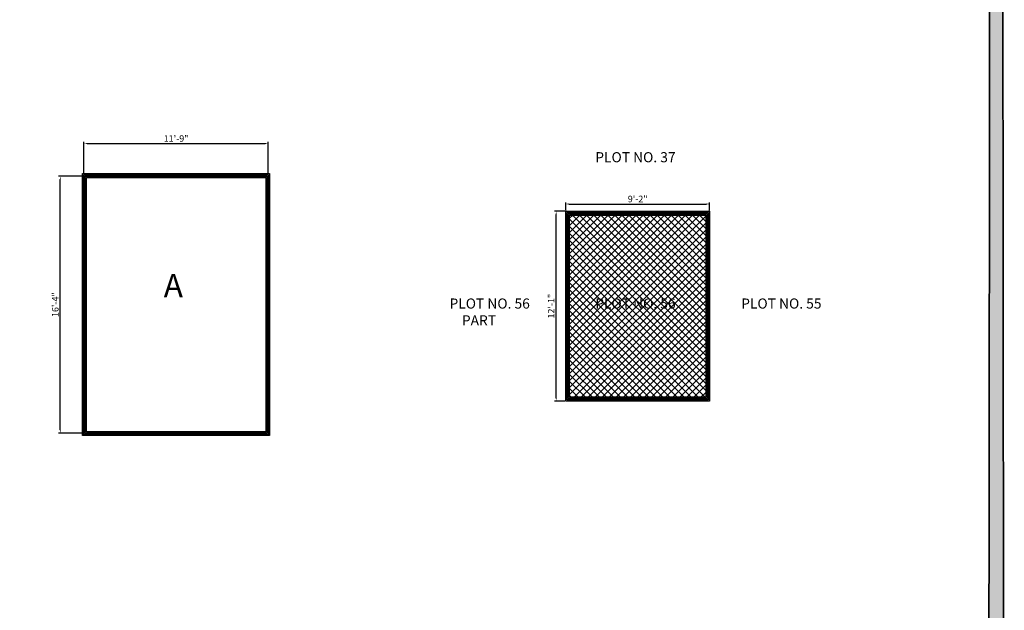
# Model space of a CAD drawing. Units: inches. Extents: x 1804 to 3296, y 909 to 2477.
# Tile 25 of 31: x 2543 to 3296, y 1449 to 1900. Entities that reach past the tile are written whole.
import ezdxf

# ---------------------------------------------------------------- set-up
doc = ezdxf.new("R2010")
doc.units = ezdxf.units.IN
for name, color, linetype, lineweight in [('A-ANNO-DIMS', 2, 'Continuous', 18), ('A-ANNO-TTLB', 156, 'Continuous', 35), ('A-WALL-PATT', 10, 'Continuous', 13), ('C-PROP', 7, 'Continuous', 25), ('C-PROP-PATT', 85, 'Continuous', 13), ('TEXT', 190, 'Continuous', 18)]:
    doc.layers.add(name, color=color, linetype=linetype, lineweight=lineweight)
doc.styles.get("Standard").update_dxf_attribs({"font": 'arial.ttf'})
doc.dimstyles.new('ISO-25', dxfattribs={"dimtxt": 5, "dimasz": 2.5, "dimexe": 1.25, "dimexo": 0.625, "dimtad": 1, "dimdec": 0, "dimlunit": 4, "dimtxsty": 'Standard', "dimcen": 2.5, "dimadec": 0, "dimazin": 0, "dimtfac": 1, "dimtdec": 0, "dimtmove": 0, "dimatfit": 3, "dimfxl": 1, "dimarcsym": 0})

# ---------------------------------------------------------------- blocks, each defined once
blk = doc.blocks.new('*D36')
at = {"layer": 'A-ANNO-DIMS', "color": 0, "lineweight": -2, "transparency": 16777216}
for p, q in [((2592.54, 1782.01), (2592.54, 1806.64)), ((2733.5, 1782.01), (2733.5, 1806.64)), ((2595.04, 1805.39), (2731, 1805.39))]:
    blk.add_line(p, q, dxfattribs=at)
at = {"layer": 'A-ANNO-DIMS', "color": 0, "lineweight": 100, "transparency": 16777216}
for points in [[(2595.04, 1805.81), (2595.04, 1804.97), (2592.54, 1805.39)], [(2731, 1805.81), (2731, 1804.97), (2733.5, 1805.39)]]:
    blk.add_solid(points, dxfattribs=at)
at = {"layer": 'Defpoints', "color": 0, "lineweight": 100, "transparency": 16777216}
for p in [(2733.5, 1805.39), (2592.54, 1781.39), (2733.5, 1781.39)]:
    blk.add_point(p, dxfattribs=at)
at = {"layer": 'A-ANNO-DIMS', "color": 0, "transparency": 16777216, "insert": (2663.02, 1808.57), "char_height": 5, "attachment_point": 5}
blk.add_mtext('11\'-9"', dxfattribs=at)
blk = doc.blocks.new('*D37')
at = {"layer": 'A-ANNO-DIMS', "color": 0, "lineweight": -2, "transparency": 16777216}
for p, q in [((2592.91, 1780.39), (2573.24, 1780.39)), ((2574.49, 1586.59), (2574.49, 1777.89)), ((2592.91, 1584.09), (2573.24, 1584.09))]:
    blk.add_line(p, q, dxfattribs=at)
at = {"layer": 'A-ANNO-DIMS', "color": 0, "lineweight": 100, "transparency": 16777216}
for points in [[(2574.08, 1777.89), (2574.91, 1777.89), (2574.49, 1780.39)], [(2574.08, 1586.59), (2574.91, 1586.59), (2574.49, 1584.09)]]:
    blk.add_solid(points, dxfattribs=at)
at = {"layer": 'Defpoints', "color": 0, "lineweight": 100, "transparency": 16777216}
for p in [(2574.49, 1780.39), (2593.54, 1780.39), (2593.54, 1584.09)]:
    blk.add_point(p, dxfattribs=at)
at = {"layer": 'A-ANNO-DIMS', "color": 0, "transparency": 16777216, "insert": (2571.31, 1682.24), "char_height": 5, "attachment_point": 5, "rotation": 90}
blk.add_mtext('16\'-4"', dxfattribs=at)
blk = doc.blocks.new('*D38')
at = {"layer": 'A-ANNO-DIMS', "color": 0, "lineweight": -2, "transparency": 16777216}
for p, q in [((2960.24, 1753.62), (2952.33, 1753.62)), ((2953.58, 1610.99), (2953.58, 1751.12)), ((2960.24, 1608.49), (2952.33, 1608.49))]:
    blk.add_line(p, q, dxfattribs=at)
at = {"layer": 'A-ANNO-DIMS', "color": 0, "lineweight": 100, "transparency": 16777216}
for points in [[(2953.16, 1751.12), (2954, 1751.12), (2953.58, 1753.62)], [(2953.16, 1610.99), (2954, 1610.99), (2953.58, 1608.49)]]:
    blk.add_solid(points, dxfattribs=at)
at = {"layer": 'Defpoints', "color": 0, "lineweight": 100, "transparency": 16777216}
for p in [(2953.58, 1753.62), (2960.87, 1753.62), (2960.87, 1608.49)]:
    blk.add_point(p, dxfattribs=at)
at = {"layer": 'A-ANNO-DIMS', "color": 0, "transparency": 16777216, "insert": (2950.44, 1681.06), "char_height": 5, "attachment_point": 5, "rotation": 90}
blk.add_mtext('12\'-1"', dxfattribs=at)
blk = doc.blocks.new('*D39')
at = {"layer": 'A-ANNO-DIMS', "color": 0, "lineweight": -2, "transparency": 16777216}
for p, q in [((2960.87, 1754.25), (2960.87, 1760.42)), ((2963.37, 1759.17), (3068.4, 1759.17)), ((3070.9, 1754.25), (3070.9, 1760.42))]:
    blk.add_line(p, q, dxfattribs=at)
at = {"layer": 'A-ANNO-DIMS', "color": 0, "lineweight": 100, "transparency": 16777216}
for points in [[(2963.37, 1759.59), (2963.37, 1758.76), (2960.87, 1759.17)], [(3068.4, 1759.59), (3068.4, 1758.76), (3070.9, 1759.17)]]:
    blk.add_solid(points, dxfattribs=at)
at = {"layer": 'Defpoints', "color": 0, "lineweight": 100, "transparency": 16777216}
for p in [(3070.9, 1759.17), (2960.87, 1753.62), (3070.9, 1753.62)]:
    blk.add_point(p, dxfattribs=at)
at = {"layer": 'A-ANNO-DIMS', "color": 0, "transparency": 16777216, "insert": (3015.89, 1762.35), "char_height": 5, "attachment_point": 5}
blk.add_mtext('9\'-2"', dxfattribs=at)

msp = doc.modelspace()

# ---------------------------------------------------------------- hatches: boundary and pattern name
at = {"layer": 'A-ANNO-TTLB'}
h = msp.add_hatch(color=256, dxfattribs=at)
h.dxf.hatch_style = 1
h.paths.add_polyline_path([(3294.53, 2476.54), (1803.79, 2476.54), (1805.43, 909.47), (3296.17, 909.47)])
h.paths.add_polyline_path([(1811, 914.33), (1812.79, 2467.54), (3285.53, 2467.54), (3283.74, 914.33)], flags=16)
h.paths.add_polyline_path([(1925.58, 1062.77), (1925.58, 1138.07), (1925.58, 1539.88), (1925.58, 1793.38), (1925.58, 1830.04), (2325.54, 1830.04), (2325.54, 1793.38), (2325.54, 1586.42), (2325.54, 1138.07), (2325.54, 1062.77)], flags=0)
h.paths.add_polyline_path([(1997.22, 1029.4), (2008.85, 1037.96), (2008.85, 1020.84)], flags=0)
h.paths.add_polyline_path([(1934.58, 1138.07), (1934.58, 1147.07), (2078.77, 1147.07), (2078.77, 1138.07), (2060.94, 1138.07)], flags=0)
h.paths.add_polyline_path([(1944.35, 1138.07), (1944.35, 1147.07), (2056.05, 1147.07), (2056.05, 1138.07)], flags=0)
h.paths.add_polyline_path([(2222.24, 1037.96), (2233.87, 1029.4), (2222.24, 1020.84)], flags=0)
h.paths.add_polyline_path([(2061.94, 1139.07), (2061.94, 1146.07), (2077.77, 1146.07), (2077.77, 1139.07)], flags=0)
h.paths.add_polyline_path([(2149.58, 1138.07), (2149.58, 1269.44), (2158.58, 1269.44), (2158.58, 1326.69), (2149.58, 1326.69), (2149.58, 1340.94), (2139.6, 1340.94), (2139.6, 1434.25), (2149.58, 1434.25), (2149.58, 1447.36), (2158.58, 1447.36), (2158.58, 1423.87), (2158.58, 1408.06), (2198.46, 1408.06), (2198.46, 1412.56), (2282.65, 1412.56), (2282.65, 1465.94), (2316.54, 1465.94), (2316.54, 1590.92), (2192.86, 1590.92), (2192.86, 1595.3), (2291.17, 1595.3), (2291.17, 1590.92), (2316.54, 1590.92), (2316.54, 1784.38), (2300.24, 1784.38), (2300.24, 1757.47), (2268, 1757.47), (2268, 1681.04), (2180.87, 1681.04), (2180.87, 1757.47), (2148.63, 1757.47), (2148.63, 1784.38), (2119.08, 1784.38), (2119.08, 1585.58), (2114.58, 1585.58), (2114.58, 1784.38), (2064.11, 1784.38), (2046.28, 1784.38), (2046.28, 1760.38), (1958.58, 1760.38), (1958.58, 1664.38), (1934.58, 1664.38), (1934.58, 1784.38), (1934.58, 1793.38), (2046.28, 1793.38), (2064.11, 1793.38), (2119.08, 1793.38), (2230.78, 1793.38), (2230.78, 1784.38), (2268, 1784.38), (2300.24, 1784.38), (2316.54, 1784.38), (2316.54, 1590.92), (2316.54, 1373.73), (2316.54, 1138.07)], flags=0)
h.paths.add_polyline_path([(2209.19, 1166.63), (2209.19, 1175.63), (2158.58, 1175.63), (2209.19, 1223.63), (2209.19, 1231.63), (2183.88, 1231.63), (2183.88, 1301.66), (2242.59, 1301.66), (2242.59, 1326.69), (2316.54, 1326.69), (2272.59, 1271.63), (2272.59, 1223.63), (2316.54, 1175.63), (2272.59, 1175.63), (2272.59, 1166.63)], flags=0)
h.paths.add_polyline_path([(1947.77, 1345.22), (1947.77, 1457.48), (1991.2, 1457.48), (1991.2, 1451.7), (1991.2, 1352.18), (1991.2, 1345.22)], flags=0)
h.paths.add_polyline_path([(2209.19, 1271.63), (2262.59, 1271.63), (2262.59, 1311.85), (2272.59, 1301.66), (2272.59, 1271.63), (2269.92, 1269.63), (2270.59, 1269.63), (2270.59, 1225.63), (2211.19, 1225.63), (2211.19, 1269.63), (2211.86, 1269.63)], flags=0)
h.paths.add_polyline_path([(2000.34, 1378.21), (2000.34, 1429.71), (2025.22, 1429.71), (2025.22, 1378.21)], flags=0)
h.paths.add_polyline_path([(2001.34, 1379.21), (2001.34, 1428.71), (2024.22, 1428.71), (2024.22, 1379.21)], flags=0)
h.paths.add_polyline_path([(2012.34, 1390.21), (2012.34, 1417.71), (2013.22, 1417.71), (2013.22, 1390.21)], flags=0)
h.paths.add_polyline_path([(2237.56, 1331.19), (2237.56, 1340.18), (2238.62, 1340.18), (2238.62, 1386.84), (2241.04, 1386.84), (2242.06, 1386.84), (2242.06, 1408.06), (2316.54, 1331.19)], flags=0)
h.paths.add_polyline_path([(1953.73, 1464.35), (1953.73, 1498.59), (1981.74, 1498.59), (1981.74, 1464.35)], flags=0)
h.paths.add_polyline_path([(1987.63, 1462.08), (1987.63, 1500.95), (2104.07, 1500.95), (2104.07, 1462.08), (2099.27, 1462.08), (1993.6, 1462.08)], flags=0)
h.paths.add_polyline_path([(1956.06, 1481.47, -1), (1979.41, 1481.47, -1)], flags=0)
edge = h.paths.add_edge_path(flags=0)
edge.add_ellipse((2299.53, 1438.37), major_axis=(0.31, 21.36), ratio=0.670333, start_angle=0, end_angle=360)
h.paths.add_polyline_path([(2297.39, 1438.37, -1), (2301.67, 1438.37, -1)], flags=0)
h.paths.add_polyline_path([(2591.54, 1163.23), (2591.54, 1179.38), (2591.54, 1379.68), (2591.54, 1395.84), (2734.5, 1395.84), (2734.5, 1379.68), (2734.5, 1179.38), (2734.5, 1163.23)], flags=0)
h.paths.add_polyline_path([(2592.54, 1164.23), (2592.54, 1166.23), (2733.5, 1166.23), (2733.5, 1164.23)], flags=0)
h.paths.add_polyline_path([(2592.54, 1180.38), (2592.54, 1378.68), (2733.5, 1378.68), (2733.5, 1180.38)], flags=0)
h.paths.add_polyline_path([(2593.54, 1181.38), (2593.54, 1377.68), (2732.5, 1377.68), (2732.5, 1181.38)], flags=0)
h.paths.add_polyline_path([(2594.54, 1182.38), (2594.54, 1376.68), (2731.5, 1376.68), (2731.5, 1182.38)], flags=0)
h.paths.add_polyline_path([(1936.95, 1697.46), (1936.95, 1736.46), (1955.41, 1736.46), (1955.41, 1697.46)], flags=0)
h.paths.add_polyline_path([(1938.48, 1718.36), (1938.48, 1734.92), (1953.65, 1734.92), (1953.65, 1718.36)], flags=0)
h.paths.add_polyline_path([(1944.75, 1726.64, -1), (1947.37, 1726.64, -1)], flags=0)
h.paths.add_polyline_path([(2592.54, 1394.84), (2733.5, 1394.84), (2733.5, 1392.84), (2592.54, 1392.84)], flags=0)
h.paths.add_polyline_path([(1976.61, 1762.5), (1976.61, 1781.44), (2012.79, 1781.44), (2012.79, 1762.5)], flags=0)
h.paths.add_polyline_path([(1979.57, 1771.97, -1), (1991.39, 1771.97, -1)], flags=0)
h.paths.add_polyline_path([(1995.36, 1771.97, -1), (2007.18, 1771.97, -1)], flags=0)
h.paths.add_polyline_path([(2251.51, 1744.53), (2268, 1730.05), (2251.51, 1730.05)], flags=0)
h.paths.add_polyline_path([(2047.28, 1785.38), (2047.28, 1792.38), (2063.11, 1792.38), (2063.11, 1785.38)], flags=0)
h.paths.add_polyline_path([(2155.08, 1770.92, -1), (2174.42, 1770.92, -1)], flags=0)
h.paths.add_polyline_path([(2188.59, 1758.27), (2188.59, 1772.81), (2222.3, 1772.81), (2222.3, 1758.27)], flags=0)
h.paths.add_polyline_path([(2223.97, 1758.27), (2223.97, 1772.81), (2257.68, 1772.81), (2257.68, 1758.27)], flags=0)
h.paths.add_polyline_path([(2274.45, 1770.92, -1), (2293.8, 1770.92, -1)], flags=0)
h.paths.add_polyline_path([(2591.54, 1582.09), (2591.54, 1782.39), (2734.5, 1782.39), (2734.5, 1582.09)], flags=0)
h.paths.add_polyline_path([(2592.54, 1583.09), (2592.54, 1781.39), (2733.5, 1781.39), (2733.5, 1583.09)], flags=0)
h.paths.add_polyline_path([(2593.54, 1584.09), (2593.54, 1780.39), (2732.5, 1780.39), (2732.5, 1584.09)], flags=0)
h.paths.add_polyline_path([(2594.54, 1585.09), (2594.54, 1779.39), (2731.5, 1779.39), (2731.5, 1585.09)], flags=0)
h.paths.add_polyline_path([(1922.17, 1978.79), (1922.17, 2295.08), (1922.17, 2296.08), (2115.67, 2296.08), (2115.67, 2384.31), (2115.67, 2385.31), (2322.12, 2385.31), (2323.12, 2385.31), (2323.12, 1979.79), (2323.12, 1978.79), (1923.17, 1978.79)], flags=0)
h.paths.add_polyline_path([(1922.17, 1978.79), (1922.17, 2051.31), (1922.17, 2214.86), (1922.17, 2296.08), (2115.67, 2296.08), (2115.67, 2385.31), (2323.12, 2385.31), (2323.12, 2280.42), (2323.12, 1978.79), (2115.67, 1978.79)], flags=0)
h.paths.add_polyline_path([(1923.17, 1979.79), (1923.17, 2050.31), (2115.67, 2050.31), (2115.67, 2051.31), (1923.17, 2051.31), (1923.17, 2213.86), (1923.17, 2214.86), (1923.17, 2295.08), (1990.02, 2295.08), (1990.02, 2214.86), (1991.02, 2214.86), (1991.02, 2295.08), (2115.67, 2295.08), (2115.67, 1979.79), (2116.67, 1979.79), (2116.67, 2304.18), (2116.67, 2384.31), (2322.12, 2384.31), (2322.12, 2280.42), (2322.12, 1979.79), (2115.67, 1979.79)], flags=0)
h.paths.add_polyline_path([(2972.46, 1192.5), (2972.46, 1196.92), (2995.47, 1196.92), (2995.47, 1255.47), (2995.09, 1255.47), (2987.42, 1249.39), (2980.08, 1255.47), (2978.05, 1255.47), (2978.05, 1257.24), (2995.47, 1257.24), (2995.47, 1261.58), (3015.37, 1261.58), (3015.37, 1333.28), (3015.37, 1414.4), (3032.82, 1414.4), (3032.82, 1333.28), (3032.82, 1261.58), (3052.66, 1261.58), (3052.66, 1255.47), (3079.86, 1255.47), (3078.72, 1254.57), (3081.47, 1252.29), (3078.56, 1249.99), (3075.81, 1252.26), (3072.57, 1249.69), (3070.36, 1251.52), (3067.67, 1249.39), (3060.34, 1255.47), (3052.66, 1255.47), (3052.66, 1196.92), (3054.58, 1196.92), (3074, 1196.92), (3074, 1192.5), (3052.66, 1192.5), (2995.47, 1192.5)], flags=0)
h.paths.add_polyline_path([(2490.75, 1979.27), (2490.75, 1980.27), (2596.87, 1980.27), (2596.87, 2051.8), (2596.87, 2052.8), (2596.87, 2216.35), (2596.87, 2297.57), (2717.32, 2297.57), (2710.57, 2305.62), (2724.07, 2305.62), (2717.32, 2297.57), (2782.37, 2297.57), (2782.37, 2395.8), (3006.82, 2395.8), (3006.82, 1981.27), (3093.73, 1981.27), (3093.73, 1980.27), (3047.51, 1980.27), (3046.37, 1979.37), (3049.11, 1977.1), (3046.2, 1974.79), (3043.46, 1977.07), (3040.21, 1974.49), (3038, 1976.32), (3035.32, 1974.2), (3027.98, 1980.27), (2871.83, 1980.27), (2871.83, 1981.27), (2791.37, 1981.27), (2791.37, 2050.8), (2597.87, 2050.8), (2597.87, 1980.27), (2597.87, 1979.27), (2546.27, 1979.27), (2545.12, 1978.37), (2547.87, 1976.1), (2544.96, 1973.79), (2542.22, 1976.07), (2538.97, 1973.49), (2536.76, 1975.32), (2534.07, 1973.2), (2526.74, 1979.27)], flags=0)
h.paths.add_polyline_path([(2597.87, 2051.8), (2606.87, 2051.8), (2606.87, 2258.39), (2597.87, 2258.39), (2597.87, 2296.57), (2606.87, 2296.57), (2606.87, 2262.39), (2782.37, 2262.39), (2782.37, 2296.57), (2790.37, 2296.57), (2790.37, 2262.39), (2791.37, 2262.39), (2791.37, 2305.67), (2791.37, 2385.8), (2996.82, 2385.8), (2996.82, 2339.85), (3006.82, 2339.85), (3006.82, 2250.12), (2997.82, 2250.12), (2997.82, 1981.27), (2996.82, 1981.27), (2872.83, 1981.27), (2872.83, 1991.8), (2871.83, 1991.8), (2871.83, 2050.8), (2790.37, 2050.8), (2597.87, 2050.8)], flags=0)
h.paths.add_polyline_path([(2179.93, 2153.92), (2179.93, 2353.97), (2259.98, 2353.97), (2259.98, 2153.92)], flags=0)
h.paths.add_polyline_path([(2180.93, 2154.92), (2180.93, 2352.97), (2258.98, 2352.97), (2258.98, 2154.92)], flags=0)
h.paths.add_polyline_path([(2960.87, 1608.49), (2960.87, 1753.62), (3070.9, 1753.62), (3070.9, 1608.49)], flags=0)
h.paths.add_polyline_path([(2961.87, 1609.49), (2961.87, 1752.62), (3069.9, 1752.62), (3069.9, 1609.49)], flags=0)
h.paths.add_polyline_path([(2962.87, 1610.49), (2962.87, 1751.62), (3068.9, 1751.62), (3068.9, 1610.49)], flags=0)
h.paths.add_polyline_path([(2963.87, 1611.49), (2963.87, 1750.62), (3067.9, 1750.62), (3067.9, 1611.49)], flags=0)
h.paths.add_polyline_path([(2782.37, 2051.8), (2782.37, 2216.32), (2791.37, 2216.32), (2791.37, 2051.8), (2872.83, 2051.8), (2872.83, 2068.56), (2884.67, 2068.56), (2884.67, 2085.33), (2896.51, 2085.33), (2896.51, 2102.09), (2908.36, 2102.09), (2908.36, 2118.85), (2920.2, 2118.85), (2920.2, 2135.62), (2932.05, 2135.62), (2932.05, 2145.3), (2925.08, 2145.3), (2925.08, 2203.2), (2996.82, 2203.2), (2996.82, 2145.3), (2953.82, 2145.3), (2872.83, 2051.8), (2790.37, 2051.8)], flags=0)
h.paths.add_polyline_path([(2717.32, 2238.65), (2710.57, 2246.7), (2724.07, 2246.7)], flags=0)
h.paths.add_polyline_path([(2003.09, 1122.79), (2017.16, 1122.79), (2017.16, 1138.74), (2003.09, 1138.74)], flags=8)
h.paths.add_polyline_path([(2174.76, 1792.72), (2188.83, 1792.72), (2188.83, 1808.66), (2174.76, 1808.66)], flags=8)
h.paths.add_polyline_path([(1987.95, 1792.51), (2002.02, 1792.51), (2002.02, 1808.45), (1987.95, 1808.45)], flags=8)
h.paths.add_polyline_path([(2148.79, 1289.26), (2160.46, 1289.26), (2160.46, 1305.2), (2148.79, 1305.2)], flags=8)
h.paths.add_polyline_path([(2115.36, 1133.57), (2127.04, 1133.57), (2127.04, 1149.51), (2115.36, 1149.51)], flags=8)
h.paths.add_polyline_path([(2237.58, 1421.48), (2249.25, 1421.48), (2249.25, 1437.43), (2237.58, 1437.43)], flags=8)
h.paths.add_polyline_path([(2134.99, 1584.32), (2146.66, 1584.32), (2146.66, 1600.26), (2134.99, 1600.26)], flags=8)
h.paths.add_polyline_path([(2101.95, 1557.31), (2113.62, 1557.31), (2113.62, 1573.25), (2101.95, 1573.25)], flags=8)
h.paths.add_polyline_path([(2937.85, 1156.77), (3120.41, 1156.77), (3120.41, 1185.72), (2937.85, 1185.72)], flags=8)
h.paths.add_polyline_path([(2980.71, 1786.71), (3050.06, 1786.71), (3050.06, 1802.66), (2980.71, 1802.66)], flags=8)
h.paths.add_polyline_path([(2869.28, 1661.96), (2938.62, 1661.96), (2938.62, 1690.8), (2869.28, 1690.8)], flags=8)
h.paths.add_polyline_path([(3092.27, 1674.86), (3161.62, 1674.86), (3161.62, 1690.8), (3092.27, 1690.8)], flags=8)
h.paths.add_polyline_path([(2980.71, 1674.86), (3050.06, 1674.86), (3050.06, 1690.8), (2980.71, 1690.8)], flags=8)
h.paths.add_polyline_path([(2649.07, 1678.23), (2674.53, 1678.23), (2674.53, 1714.76), (2649.07, 1714.76)], flags=8)
h.paths.add_polyline_path([(2530.84, 1981.63), (2549.13, 1981.63), (2549.13, 1997.57), (2530.84, 1997.57)], flags=8)
h.paths.add_polyline_path([(3031.29, 1981.77), (3049.58, 1981.77), (3049.58, 1997.71), (3031.29, 1997.71)], flags=8)
h.paths.add_polyline_path([(2715.38, 1911.9), (2851.54, 1911.9), (2851.54, 1940.85), (2715.38, 1940.85)], flags=8)
h.paths.add_polyline_path([(2015.23, 1927.36), (2205.42, 1927.36), (2205.42, 1956.3), (2015.23, 1956.3)], flags=8)
h.paths.add_polyline_path([(2671.84, 2057.84), (2702.75, 2057.84), (2702.75, 2073.79), (2671.84, 2073.79)], flags=8)
h.paths.add_polyline_path([(2678.5, 2316.52), (2765.26, 2316.52), (2765.26, 2332.46), (2678.5, 2332.46)], flags=8)
h.paths.add_polyline_path([(2678.48, 2271.96), (2736.41, 2271.96), (2736.41, 2287.9), (2678.48, 2287.9)], flags=8)
h.paths.add_polyline_path([(2019.2, 972.79), (2243.21, 972.79), (2243.21, 1001.74), (2019.2, 1001.74)], flags=8)
h.paths.add_polyline_path([(2097.06, 1021.56), (2132.16, 1021.56), (2132.16, 1037.51), (2097.06, 1037.51)], flags=8)
h.paths.add_polyline_path([(2182.47, 1360.48), (2207.35, 1360.48), (2207.35, 1376.42), (2182.47, 1376.42)], flags=8)
h.paths.add_polyline_path([(2261.12, 1361.77), (2295.01, 1361.77), (2295.01, 1377.71), (2261.12, 1377.71)], flags=8)
h.paths.add_polyline_path([(2245.75, 1511.51), (2278.44, 1511.51), (2278.44, 1527.46), (2245.75, 1527.46)], flags=8)
h.paths.add_polyline_path([(1991.16, 1296.29), (2060.51, 1296.29), (2060.51, 1312.23), (1991.16, 1312.23)], flags=8)
h.paths.add_polyline_path([(2187, 1651.35), (2246.71, 1651.35), (2246.71, 1667.29), (2187, 1667.29)], flags=8)
h.paths.add_polyline_path([(1976.49, 1684.81), (2068.63, 1684.81), (2068.63, 1700.76), (1976.49, 1700.76)], flags=8)
at = {"layer": 'A-WALL-PATT'}
h = msp.add_hatch(color=256, dxfattribs=at)
h.dxf.hatch_style = 1
h.paths.add_polyline_path([(2119.08, 1544.38), (1925.58, 1544.38), (1925.58, 1539.88), (2119.08, 1539.88)])
h.paths.add_polyline_path([(2119.08, 1545.58), (2114.58, 1545.58), (2114.58, 1544.38), (2119.08, 1544.38)])
h.paths.add_polyline_path([(1965.87, 1658.79), (1965.87, 1679.09), (1955.57, 1679.09), (1955.57, 1658.79)], flags=9)
h.paths.add_polyline_path([(2293.18, 1677.29), (2293.18, 1697.58), (2282.88, 1697.58), (2282.88, 1677.29)], flags=9)
h.paths.add_polyline_path([(2271.13, 1545.23), (2287.53, 1545.23), (2287.53, 1555.53), (2271.13, 1555.53)], flags=9)
h.paths.add_polyline_path([(2303.26, 1488.52), (2303.26, 1508.82), (2292.95, 1508.82), (2292.95, 1488.52)], flags=9)
h.paths.add_polyline_path([(2271.13, 1393.15), (2287.53, 1393.15), (2287.53, 1403.45), (2271.13, 1403.45)], flags=9)
h.paths.add_polyline_path([(2306.48, 1361.45), (2306.48, 1377.86), (2296.18, 1377.86), (2296.18, 1361.45)], flags=9)
h.paths.add_polyline_path([(2174.54, 1361.45), (2174.54, 1377.86), (2164.23, 1377.86), (2164.23, 1361.45)], flags=9)
h.paths.add_polyline_path([(1968.21, 1333.34), (1968.21, 1353.64), (1957.91, 1353.64), (1957.91, 1333.34)], flags=9)
h.paths.add_polyline_path([(2003.09, 1122.79), (2017.16, 1122.79), (2017.16, 1138.74), (2003.09, 1138.74)], flags=9)
h.paths.add_polyline_path([(2174.76, 1792.72), (2188.83, 1792.72), (2188.83, 1808.66), (2174.76, 1808.66)], flags=9)
h.paths.add_polyline_path([(1987.95, 1792.51), (2002.02, 1792.51), (2002.02, 1808.45), (1987.95, 1808.45)], flags=9)
h.paths.add_polyline_path([(2148.79, 1289.26), (2160.46, 1289.26), (2160.46, 1305.2), (2148.79, 1305.2)], flags=9)
h.paths.add_polyline_path([(2115.36, 1133.57), (2127.04, 1133.57), (2127.04, 1149.51), (2115.36, 1149.51)], flags=9)
h.paths.add_polyline_path([(2237.58, 1421.48), (2249.25, 1421.48), (2249.25, 1437.43), (2237.58, 1437.43)], flags=9)
h.paths.add_polyline_path([(2134.99, 1584.32), (2146.66, 1584.32), (2146.66, 1600.26), (2134.99, 1600.26)], flags=9)
h.paths.add_polyline_path([(2101.95, 1557.31), (2113.62, 1557.31), (2113.62, 1573.25), (2101.95, 1573.25)], flags=9)
h.paths.add_polyline_path([(2937.85, 1156.77), (3120.41, 1156.77), (3120.41, 1185.72), (2937.85, 1185.72)], flags=9)
h.paths.add_polyline_path([(2980.71, 1786.71), (3050.06, 1786.71), (3050.06, 1802.66), (2980.71, 1802.66)], flags=9)
h.paths.add_polyline_path([(2869.28, 1661.96), (2938.62, 1661.96), (2938.62, 1690.8), (2869.28, 1690.8)], flags=9)
h.paths.add_polyline_path([(3092.27, 1674.86), (3161.62, 1674.86), (3161.62, 1690.8), (3092.27, 1690.8)], flags=9)
h.paths.add_polyline_path([(2980.71, 1674.86), (3050.06, 1674.86), (3050.06, 1690.8), (2980.71, 1690.8)], flags=9)
h.paths.add_polyline_path([(2649.07, 1678.23), (2674.53, 1678.23), (2674.53, 1714.76), (2649.07, 1714.76)], flags=9)
h.paths.add_polyline_path([(2530.84, 1981.63), (2549.13, 1981.63), (2549.13, 1997.57), (2530.84, 1997.57)], flags=9)
h.paths.add_polyline_path([(3031.29, 1981.77), (3049.58, 1981.77), (3049.58, 1997.71), (3031.29, 1997.71)], flags=9)
h.paths.add_polyline_path([(2715.38, 1911.9), (2851.54, 1911.9), (2851.54, 1940.85), (2715.38, 1940.85)], flags=9)
h.paths.add_polyline_path([(2015.23, 1927.36), (2205.42, 1927.36), (2205.42, 1956.3), (2015.23, 1956.3)], flags=9)
h.paths.add_polyline_path([(2671.84, 2057.84), (2702.75, 2057.84), (2702.75, 2073.79), (2671.84, 2073.79)], flags=9)
h.paths.add_polyline_path([(2678.5, 2316.52), (2765.26, 2316.52), (2765.26, 2332.46), (2678.5, 2332.46)], flags=9)
h.paths.add_polyline_path([(2678.48, 2271.96), (2736.41, 2271.96), (2736.41, 2287.9), (2678.48, 2287.9)], flags=9)
h.paths.add_polyline_path([(2019.2, 972.79), (2243.21, 972.79), (2243.21, 1001.74), (2019.2, 1001.74)], flags=9)
h.paths.add_polyline_path([(2097.06, 1021.56), (2132.16, 1021.56), (2132.16, 1037.51), (2097.06, 1037.51)], flags=9)
h.paths.add_polyline_path([(2182.47, 1360.48), (2207.35, 1360.48), (2207.35, 1376.42), (2182.47, 1376.42)], flags=9)
h.paths.add_polyline_path([(2261.12, 1361.77), (2295.01, 1361.77), (2295.01, 1377.71), (2261.12, 1377.71)], flags=9)
h.paths.add_polyline_path([(2245.75, 1511.51), (2278.44, 1511.51), (2278.44, 1527.46), (2245.75, 1527.46)], flags=9)
h.paths.add_polyline_path([(1991.16, 1296.29), (2060.51, 1296.29), (2060.51, 1312.23), (1991.16, 1312.23)], flags=9)
h.paths.add_polyline_path([(2187, 1651.35), (2246.71, 1651.35), (2246.71, 1667.29), (2187, 1667.29)], flags=9)
h.paths.add_polyline_path([(1976.49, 1684.81), (2068.63, 1684.81), (2068.63, 1700.76), (1976.49, 1700.76)], flags=9)
h = msp.add_hatch(color=256, dxfattribs=at)
h.dxf.hatch_style = 1
h.paths.add_polyline_path([(2149.58, 1147.07), (2141.21, 1147.07), (2141.21, 1144.07), (2141.21, 1138.07), (2149.58, 1138.07)])
h.paths.add_polyline_path([(2101.21, 1144.07, -0.01877), (2101.32, 1147.07), (2078.77, 1147.07), (2078.77, 1138.07), (2101.21, 1138.07)])
h.paths.add_polyline_path([(2060.94, 1147.07), (2056.05, 1147.07), (2056.05, 1138.07), (2060.94, 1138.07)])
h.paths.add_polyline_path([(1944.35, 1147.07), (1934.58, 1147.07), (1934.58, 1138.07), (1944.35, 1138.07)])
h.paths.add_polyline_path([(2158.58, 1269.44), (2149.58, 1269.44), (2149.58, 1138.07), (2158.58, 1138.07)])
h.paths.add_polyline_path([(2003.09, 1122.79), (2017.16, 1122.79), (2017.16, 1138.74), (2003.09, 1138.74)], flags=9)
h.paths.add_polyline_path([(2174.76, 1792.72), (2188.83, 1792.72), (2188.83, 1808.66), (2174.76, 1808.66)], flags=9)
h.paths.add_polyline_path([(1987.95, 1792.51), (2002.02, 1792.51), (2002.02, 1808.45), (1987.95, 1808.45)], flags=9)
h.paths.add_polyline_path([(2148.79, 1289.26), (2160.46, 1289.26), (2160.46, 1305.2), (2148.79, 1305.2)], flags=9)
h.paths.add_polyline_path([(2115.36, 1133.57), (2127.04, 1133.57), (2127.04, 1149.51), (2115.36, 1149.51)], flags=9)
h.paths.add_polyline_path([(2237.58, 1421.48), (2249.25, 1421.48), (2249.25, 1437.43), (2237.58, 1437.43)], flags=9)
h.paths.add_polyline_path([(2134.99, 1584.32), (2146.66, 1584.32), (2146.66, 1600.26), (2134.99, 1600.26)], flags=9)
h.paths.add_polyline_path([(2101.95, 1557.31), (2113.62, 1557.31), (2113.62, 1573.25), (2101.95, 1573.25)], flags=9)
h.paths.add_polyline_path([(2937.85, 1156.77), (3120.41, 1156.77), (3120.41, 1185.72), (2937.85, 1185.72)], flags=9)
h.paths.add_polyline_path([(2980.71, 1786.71), (3050.06, 1786.71), (3050.06, 1802.66), (2980.71, 1802.66)], flags=9)
h.paths.add_polyline_path([(2869.28, 1661.96), (2938.62, 1661.96), (2938.62, 1690.8), (2869.28, 1690.8)], flags=9)
h.paths.add_polyline_path([(3092.27, 1674.86), (3161.62, 1674.86), (3161.62, 1690.8), (3092.27, 1690.8)], flags=9)
h.paths.add_polyline_path([(2980.71, 1674.86), (3050.06, 1674.86), (3050.06, 1690.8), (2980.71, 1690.8)], flags=9)
h.paths.add_polyline_path([(2649.07, 1678.23), (2674.53, 1678.23), (2674.53, 1714.76), (2649.07, 1714.76)], flags=9)
h.paths.add_polyline_path([(2530.84, 1981.63), (2549.13, 1981.63), (2549.13, 1997.57), (2530.84, 1997.57)], flags=9)
h.paths.add_polyline_path([(3031.29, 1981.77), (3049.58, 1981.77), (3049.58, 1997.71), (3031.29, 1997.71)], flags=9)
h.paths.add_polyline_path([(2715.38, 1911.9), (2851.54, 1911.9), (2851.54, 1940.85), (2715.38, 1940.85)], flags=9)
h.paths.add_polyline_path([(2015.23, 1927.36), (2205.42, 1927.36), (2205.42, 1956.3), (2015.23, 1956.3)], flags=9)
h.paths.add_polyline_path([(2671.84, 2057.84), (2702.75, 2057.84), (2702.75, 2073.79), (2671.84, 2073.79)], flags=9)
h.paths.add_polyline_path([(2678.5, 2316.52), (2765.26, 2316.52), (2765.26, 2332.46), (2678.5, 2332.46)], flags=9)
h.paths.add_polyline_path([(2678.48, 2271.96), (2736.41, 2271.96), (2736.41, 2287.9), (2678.48, 2287.9)], flags=9)
h.paths.add_polyline_path([(2019.2, 972.79), (2243.21, 972.79), (2243.21, 1001.74), (2019.2, 1001.74)], flags=9)
h.paths.add_polyline_path([(2097.06, 1021.56), (2132.16, 1021.56), (2132.16, 1037.51), (2097.06, 1037.51)], flags=9)
h.paths.add_polyline_path([(2182.47, 1360.48), (2207.35, 1360.48), (2207.35, 1376.42), (2182.47, 1376.42)], flags=9)
h.paths.add_polyline_path([(2261.12, 1361.77), (2295.01, 1361.77), (2295.01, 1377.71), (2261.12, 1377.71)], flags=9)
h.paths.add_polyline_path([(2245.75, 1511.51), (2278.44, 1511.51), (2278.44, 1527.46), (2245.75, 1527.46)], flags=9)
h.paths.add_polyline_path([(1991.16, 1296.29), (2060.51, 1296.29), (2060.51, 1312.23), (1991.16, 1312.23)], flags=9)
h.paths.add_polyline_path([(2187, 1651.35), (2246.71, 1651.35), (2246.71, 1667.29), (2187, 1667.29)], flags=9)
h.paths.add_polyline_path([(1976.49, 1684.81), (2068.63, 1684.81), (2068.63, 1700.76), (1976.49, 1700.76)], flags=9)
h = msp.add_hatch(color=256, dxfattribs=at)
h.dxf.hatch_style = 1
h.paths.add_polyline_path([(2158.58, 1275.49), (2155.29, 1275.49), (2149.58, 1275.49), (2149.58, 1269.44), (2158.58, 1269.44)])
h.paths.add_polyline_path([(2158.58, 1326.69), (2149.58, 1326.69), (2149.58, 1319.33), (2155.29, 1319.33), (2158.58, 1319.33)])
h.paths.add_polyline_path([(2158.58, 1402.2), (2158.58, 1423.87), (2158.58, 1447.36), (2149.58, 1447.36), (2149.58, 1423.87), (2149.58, 1340.94), (2149.58, 1326.69), (2158.58, 1326.69), (2158.58, 1354.23)])
h.paths.add_polyline_path([(1965.87, 1658.79), (1965.87, 1679.09), (1955.57, 1679.09), (1955.57, 1658.79)], flags=9)
h.paths.add_polyline_path([(2293.18, 1677.29), (2293.18, 1697.58), (2282.88, 1697.58), (2282.88, 1677.29)], flags=9)
h.paths.add_polyline_path([(2271.13, 1545.23), (2287.53, 1545.23), (2287.53, 1555.53), (2271.13, 1555.53)], flags=9)
h.paths.add_polyline_path([(2303.26, 1488.52), (2303.26, 1508.82), (2292.95, 1508.82), (2292.95, 1488.52)], flags=9)
h.paths.add_polyline_path([(2271.13, 1393.15), (2287.53, 1393.15), (2287.53, 1403.45), (2271.13, 1403.45)], flags=9)
h.paths.add_polyline_path([(2306.48, 1361.45), (2306.48, 1377.86), (2296.18, 1377.86), (2296.18, 1361.45)], flags=9)
h.paths.add_polyline_path([(2189.9, 1340.62), (2206.31, 1340.62), (2206.31, 1350.92), (2189.9, 1350.92)], flags=9)
h.paths.add_polyline_path([(2174.54, 1361.45), (2174.54, 1377.86), (2164.23, 1377.86), (2164.23, 1361.45)], flags=9)
h.paths.add_polyline_path([(2304.24, 1240.8), (2304.24, 1261.09), (2293.94, 1261.09), (2293.94, 1240.8)], flags=9)
h.paths.add_polyline_path([(2227.19, 1188.73), (2247.49, 1188.73), (2247.49, 1199.03), (2227.19, 1199.03)], flags=9)
h.paths.add_polyline_path([(2181.93, 1144.21), (2181.93, 1160.62), (2171.63, 1160.62), (2171.63, 1144.21)], flags=9)
h.paths.add_polyline_path([(1968.21, 1333.34), (1968.21, 1353.64), (1957.91, 1353.64), (1957.91, 1333.34)], flags=9)
h.paths.add_polyline_path([(2029.78, 1203.53), (2053.95, 1203.53), (2053.95, 1213.83), (2029.78, 1213.83)], flags=9)
h.paths.add_polyline_path([(2576.51, 1671.88), (2576.51, 1692.17), (2566.21, 1692.17), (2566.21, 1671.88)], flags=9)
h.paths.add_polyline_path([(2566.99, 1269.67), (2566.99, 1289.96), (2556.68, 1289.96), (2556.68, 1269.67)], flags=9)
h.paths.add_polyline_path([(2581.85, 1269.17), (2581.85, 1289.46), (2571.54, 1289.46), (2571.54, 1269.17)], flags=9)
h.paths.add_polyline_path([(2650.71, 1409.75), (2674.89, 1409.75), (2674.89, 1420.05), (2650.71, 1420.05)], flags=9)
h.paths.add_polyline_path([(2003.09, 1122.79), (2017.16, 1122.79), (2017.16, 1138.74), (2003.09, 1138.74)], flags=9)
h.paths.add_polyline_path([(2174.76, 1792.72), (2188.83, 1792.72), (2188.83, 1808.66), (2174.76, 1808.66)], flags=9)
h.paths.add_polyline_path([(1987.95, 1792.51), (2002.02, 1792.51), (2002.02, 1808.45), (1987.95, 1808.45)], flags=9)
h.paths.add_polyline_path([(2148.79, 1289.26), (2160.46, 1289.26), (2160.46, 1305.2), (2148.79, 1305.2)], flags=9)
h.paths.add_polyline_path([(2115.36, 1133.57), (2127.04, 1133.57), (2127.04, 1149.51), (2115.36, 1149.51)], flags=9)
h.paths.add_polyline_path([(2237.58, 1421.48), (2249.25, 1421.48), (2249.25, 1437.43), (2237.58, 1437.43)], flags=9)
h.paths.add_polyline_path([(2134.99, 1584.32), (2146.66, 1584.32), (2146.66, 1600.26), (2134.99, 1600.26)], flags=9)
h.paths.add_polyline_path([(2101.95, 1557.31), (2113.62, 1557.31), (2113.62, 1573.25), (2101.95, 1573.25)], flags=9)
h.paths.add_polyline_path([(2937.85, 1156.77), (3120.41, 1156.77), (3120.41, 1185.72), (2937.85, 1185.72)], flags=9)
h.paths.add_polyline_path([(2980.71, 1786.71), (3050.06, 1786.71), (3050.06, 1802.66), (2980.71, 1802.66)], flags=9)
h.paths.add_polyline_path([(2869.28, 1661.96), (2938.62, 1661.96), (2938.62, 1690.8), (2869.28, 1690.8)], flags=9)
h.paths.add_polyline_path([(3092.27, 1674.86), (3161.62, 1674.86), (3161.62, 1690.8), (3092.27, 1690.8)], flags=9)
h.paths.add_polyline_path([(2980.71, 1674.86), (3050.06, 1674.86), (3050.06, 1690.8), (2980.71, 1690.8)], flags=9)
h.paths.add_polyline_path([(2649.07, 1678.23), (2674.53, 1678.23), (2674.53, 1714.76), (2649.07, 1714.76)], flags=9)
h.paths.add_polyline_path([(2530.84, 1981.63), (2549.13, 1981.63), (2549.13, 1997.57), (2530.84, 1997.57)], flags=9)
h.paths.add_polyline_path([(3031.29, 1981.77), (3049.58, 1981.77), (3049.58, 1997.71), (3031.29, 1997.71)], flags=9)
h.paths.add_polyline_path([(2715.38, 1911.9), (2851.54, 1911.9), (2851.54, 1940.85), (2715.38, 1940.85)], flags=9)
h.paths.add_polyline_path([(2015.23, 1927.36), (2205.42, 1927.36), (2205.42, 1956.3), (2015.23, 1956.3)], flags=9)
h.paths.add_polyline_path([(2671.84, 2057.84), (2702.75, 2057.84), (2702.75, 2073.79), (2671.84, 2073.79)], flags=9)
h.paths.add_polyline_path([(2678.5, 2316.52), (2765.26, 2316.52), (2765.26, 2332.46), (2678.5, 2332.46)], flags=9)
h.paths.add_polyline_path([(2678.48, 2271.96), (2736.41, 2271.96), (2736.41, 2287.9), (2678.48, 2287.9)], flags=9)
h.paths.add_polyline_path([(2019.2, 972.79), (2243.21, 972.79), (2243.21, 1001.74), (2019.2, 1001.74)], flags=9)
h.paths.add_polyline_path([(2097.06, 1021.56), (2132.16, 1021.56), (2132.16, 1037.51), (2097.06, 1037.51)], flags=9)
h.paths.add_polyline_path([(2182.47, 1360.48), (2207.35, 1360.48), (2207.35, 1376.42), (2182.47, 1376.42)], flags=9)
h.paths.add_polyline_path([(2261.12, 1361.77), (2295.01, 1361.77), (2295.01, 1377.71), (2261.12, 1377.71)], flags=9)
h.paths.add_polyline_path([(2245.75, 1511.51), (2278.44, 1511.51), (2278.44, 1527.46), (2245.75, 1527.46)], flags=9)
h.paths.add_polyline_path([(1991.16, 1296.29), (2060.51, 1296.29), (2060.51, 1312.23), (1991.16, 1312.23)], flags=9)
h.paths.add_polyline_path([(2187, 1651.35), (2246.71, 1651.35), (2246.71, 1667.29), (2187, 1667.29)], flags=9)
h.paths.add_polyline_path([(1976.49, 1684.81), (2068.63, 1684.81), (2068.63, 1700.76), (1976.49, 1700.76)], flags=9)
at = {"layer": 'C-PROP-PATT'}
h = msp.add_hatch(color=256, dxfattribs=at)
h.dxf.hatch_style = 1
h.paths.add_polyline_path([(2591.54, 1582.09), (2734.5, 1582.09), (2734.5, 1782.39), (2591.54, 1782.39)])
h.paths.add_polyline_path([(2733.5, 1781.39), (2733.5, 1583.09), (2592.54, 1583.09), (2592.54, 1781.39)], flags=0)
h.paths.add_polyline_path([(2732.5, 1780.39), (2732.5, 1584.09), (2593.54, 1584.09), (2593.54, 1780.39)], flags=0)
h.paths.add_polyline_path([(2731.5, 1779.39), (2731.5, 1585.09), (2594.54, 1585.09), (2594.54, 1779.39)], flags=0)
h.paths.add_polyline_path([(2593.54, 1584.09), (2732.5, 1584.09), (2732.5, 1780.39), (2593.54, 1780.39)], flags=0)
h.paths.add_polyline_path([(2592.54, 1583.09), (2733.5, 1583.09), (2733.5, 1781.39), (2592.54, 1781.39)], flags=16)
h.paths.add_polyline_path([(2649.07, 1678.23), (2674.53, 1678.23), (2674.53, 1714.76), (2649.07, 1714.76)], flags=8)
h = msp.add_hatch(color=256, dxfattribs=at)
h.dxf.hatch_style = 1
h.paths.add_polyline_path([(2592.54, 1583.09), (2733.5, 1583.09), (2733.5, 1781.39), (2592.54, 1781.39)])
h.paths.add_polyline_path([(2593.54, 1584.09), (2732.5, 1584.09), (2732.5, 1780.39), (2593.54, 1780.39)], flags=16)
h.paths.add_polyline_path([(2731.5, 1779.39), (2731.5, 1585.09), (2594.54, 1585.09), (2594.54, 1779.39)], flags=0)
h.paths.add_polyline_path([(2594.54, 1585.09), (2731.5, 1585.09), (2731.5, 1779.39), (2594.54, 1779.39)], flags=0)
h.paths.add_polyline_path([(2649.07, 1678.23), (2674.53, 1678.23), (2674.53, 1714.76), (2649.07, 1714.76)], flags=8)
h = msp.add_hatch(color=256, dxfattribs=at)
h.dxf.hatch_style = 1
h.paths.add_polyline_path([(2593.54, 1584.09), (2732.5, 1584.09), (2732.5, 1780.39), (2593.54, 1780.39)])
h.paths.add_polyline_path([(2594.54, 1585.09), (2731.5, 1585.09), (2731.5, 1779.39), (2594.54, 1779.39)], flags=16)
h.paths.add_polyline_path([(2649.07, 1678.23), (2674.53, 1678.23), (2674.53, 1714.76), (2649.07, 1714.76)], flags=8)
h = msp.add_hatch(color=256, dxfattribs=at)
h.dxf.hatch_style = 1
h.paths.add_polyline_path([(2960.87, 1608.49), (3070.9, 1608.49), (3070.9, 1753.62), (2960.87, 1753.62)])
h.paths.add_polyline_path([(2961.87, 1609.49), (3069.9, 1609.49), (3069.9, 1752.62), (2961.87, 1752.62)], flags=16)
h.paths.add_polyline_path([(2962.87, 1751.62), (3068.9, 1751.62), (3068.9, 1610.49), (2962.87, 1610.49)], flags=0)
h.paths.add_polyline_path([(2963.87, 1750.62), (3067.9, 1750.62), (3067.9, 1611.49), (2963.87, 1611.49)], flags=0)
h.paths.add_polyline_path([(2962.87, 1610.49), (3068.9, 1610.49), (3068.9, 1751.62), (2962.87, 1751.62)], flags=0)
h.paths.add_polyline_path([(2980.71, 1674.86), (3050.06, 1674.86), (3050.06, 1690.8), (2980.71, 1690.8)], flags=8)
h = msp.add_hatch(color=256, dxfattribs=at)
h.dxf.hatch_style = 1
h.paths.add_polyline_path([(2961.87, 1609.49), (3069.9, 1609.49), (3069.9, 1752.62), (2961.87, 1752.62)])
h.paths.add_polyline_path([(2962.87, 1610.49), (3068.9, 1610.49), (3068.9, 1751.62), (2962.87, 1751.62)], flags=16)
h.paths.add_polyline_path([(3067.9, 1750.62), (3067.9, 1611.49), (2963.87, 1611.49), (2963.87, 1750.62)], flags=0)
h.paths.add_polyline_path([(2980.71, 1674.86), (3050.06, 1674.86), (3050.06, 1690.8), (2980.71, 1690.8)], flags=8)
h = msp.add_hatch(color=256, dxfattribs=at)
h.dxf.hatch_style = 1
h.paths.add_polyline_path([(2962.87, 1610.49), (3068.9, 1610.49), (3068.9, 1751.62), (2962.87, 1751.62)])
h.paths.add_polyline_path([(2963.87, 1611.49), (3067.9, 1611.49), (3067.9, 1750.62), (2963.87, 1750.62)], flags=16)
h.paths.add_polyline_path([(2980.71, 1674.86), (3050.06, 1674.86), (3050.06, 1690.8), (2980.71, 1690.8)], flags=8)
h = msp.add_hatch(dxfattribs=at)
h.set_pattern_fill('ANSI37', color=256, scale=1.2)
h.set_pattern_definition([(45, (0, 255.3213), (-2.694077, 2.694077), []), (135, (0, 255.3213), (-2.694077, -2.694077), [])])
h.paths.add_polyline_path([(2963.87, 1750.62), (2963.87, 1611.49), (3067.9, 1611.49), (3067.9, 1750.62)])
h.paths.add_polyline_path([(2980.71, 1674.86), (3050.06, 1674.86), (3050.06, 1690.8), (2980.71, 1690.8)], flags=24)

# ---------------------------------------------------------------- linework, layer by layer
at = {"layer": 'A-ANNO-TTLB'}
for points in [[(1803.79, 2476.54), (3294.53, 2476.54), (3296.17, 909.47), (1805.43, 909.47)], [(1812.79, 2467.54), (3285.53, 2467.54), (3283.74, 914.33), (1811, 914.33)]]:
    msp.add_lwpolyline(points, close=True, dxfattribs=at)
at = {"layer": 'C-PROP'}
for points in [[(2591.54, 1782.39), (2734.5, 1782.39), (2734.5, 1582.09), (2591.54, 1582.09)], [(2592.54, 1781.39), (2733.5, 1781.39), (2733.5, 1583.09), (2592.54, 1583.09)], [(2593.54, 1780.39), (2732.5, 1780.39), (2732.5, 1584.09), (2593.54, 1584.09)], [(2594.54, 1779.39), (2731.5, 1779.39), (2731.5, 1585.09), (2594.54, 1585.09)], [(2960.87, 1753.62), (3070.9, 1753.62), (3070.9, 1608.49), (2960.87, 1608.49)], [(2961.87, 1752.62), (3069.9, 1752.62), (3069.9, 1609.49), (2961.87, 1609.49)], [(2962.87, 1751.62), (3068.9, 1751.62), (3068.9, 1610.49), (2962.87, 1610.49)], [(2963.87, 1750.62), (3067.9, 1750.62), (3067.9, 1611.49), (2963.87, 1611.49)]]:
    msp.add_lwpolyline(points, close=True, dxfattribs=at)

# ---------------------------------------------------------------- texts
at = {"layer": 'TEXT', "attachment_point": 1}
for s, width, gutter_width, heights, insert, char_height in [('PLOT NO. 37', 163.3261, 38.69, [8.01], (2983.48, 1798.81), 7.7373), ('A', 374.2247, 88.64, [0], (2653.54, 1705.64), 17.73), ('PLOT NO. 56\\P    PART', 163.3261, 38.69, [0], (2872.04, 1686.96), 7.7373), ('PLOT NO. 56', 163.3261, 38.69, [0], (2983.48, 1686.96), 7.7373), ('PLOT NO. 55', 163.3261, 38.69, [0], (3095.04, 1686.96), 7.7373)]:
    msp.add_mtext_dynamic_manual_height_columns(s, width=width, gutter_width=gutter_width, heights=heights, dxfattribs=dict(at, insert=insert, char_height=char_height))

# ---------------------------------------------------------------- dimensions: what is measured, and where the dimension line sits
at = {"layer": 'A-ANNO-DIMS'}
for base, p1, p2, picture, middle in [((2733.5, 1805.39), (2592.54, 1781.39), (2733.5, 1781.39), '*D36', (2663.02, 1808.57)), ((3070.9, 1759.17), (2960.87, 1753.62), (3070.9, 1753.62), '*D39', (3015.89, 1762.35))]:
    dim = msp.add_linear_dim(base=base, p1=p1, p2=p2, dimstyle='ISO-25', override={"dimclrd": 0, "dimclre": 0, "dimclrt": 0}, dxfattribs=at)
    dim.commit()
    dim.dimension.update_dxf_attribs({"geometry": picture, "text_midpoint": middle})
for base, p1, p2, picture, middle in [((2574.49, 1780.39), (2593.54, 1584.09), (2593.54, 1780.39), '*D37', (2571.31, 1682.24)), ((2953.58, 1753.62), (2960.87, 1608.49), (2960.87, 1753.62), '*D38', (2950.44, 1681.06))]:
    dim = msp.add_linear_dim(base=base, p1=p1, p2=p2, angle=90, dimstyle='ISO-25', override={"dimclrd": 0, "dimclre": 0, "dimclrt": 0}, dxfattribs=at)
    dim.commit()
    dim.dimension.update_dxf_attribs({"geometry": picture, "text_midpoint": middle})

doc.saveas('drawing.dxf')
